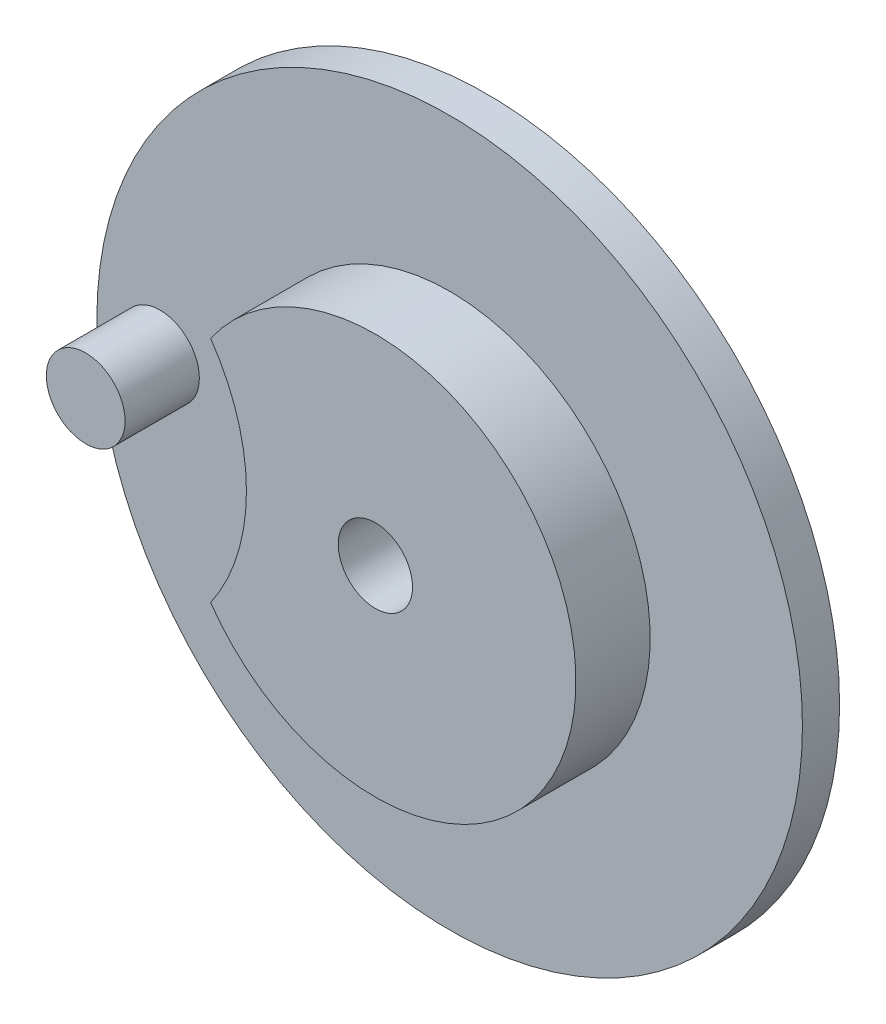
from build123d import *

# Parameters (mm, degrees)
DISC_PROFILE_R        = 47.5
DISC_95X5_DEPTH       = 5
DRIVE_PIN_PROFILE_R   = 5.3
DRIVE_PIN_10_6_DEPTH  = 10
HUB_PROFILE_R         = 27
HUB_54X10_DEPTH       = 10
HUB_START             = -10
HUB_FLAT_CUT_DEPTH    = 10
CENTRE_BORE_PROFILE_R = 5
CENTRE_BORE_10_DEPTH  = 30


with BuildPart() as part:
    # Disc Profile → Disc Ø95x5 (new body)
    with BuildSketch(Plane.XY):
        Circle(DISC_PROFILE_R)
    extrude(amount=DISC_95X5_DEPTH)

    # Drive Pin Profile → Drive Pin Ø10.6 (add)
    with BuildSketch(Plane.XY.offset(5)):
        with Locations((-39, 0)):
            Circle(DRIVE_PIN_PROFILE_R)
    extrude(amount=DRIVE_PIN_10_6_DEPTH)

    # Hub Profile → Hub Ø54x10 (add)
    with BuildSketch(Plane.XY.offset(5)):
        Circle(HUB_PROFILE_R)
    extrude(amount=HUB_54X10_DEPTH)

    # Hub Flat Profile → Hub Flat Cut (cut)
    with BuildSketch(Plane.XY.offset(15).offset(HUB_START)):
        with BuildLine():
            ThreePointArc((-22.179240987, 15.397443595), (-27, 0), (-22.179240987, -15.397443595))
            ThreePointArc((-22.179240987, -15.397443595), (-17.358481974, 0), (-22.179240987, 15.397443595))
        make_face()
    extrude(amount=HUB_FLAT_CUT_DEPTH, mode=Mode.SUBTRACT)

    # Centre Bore Profile → Centre Bore Ø10 (cut)
    with BuildSketch(Plane.XY.offset(15)):
        Circle(CENTRE_BORE_PROFILE_R)
    extrude(amount=-CENTRE_BORE_10_DEPTH, mode=Mode.SUBTRACT)


solid = part.part
